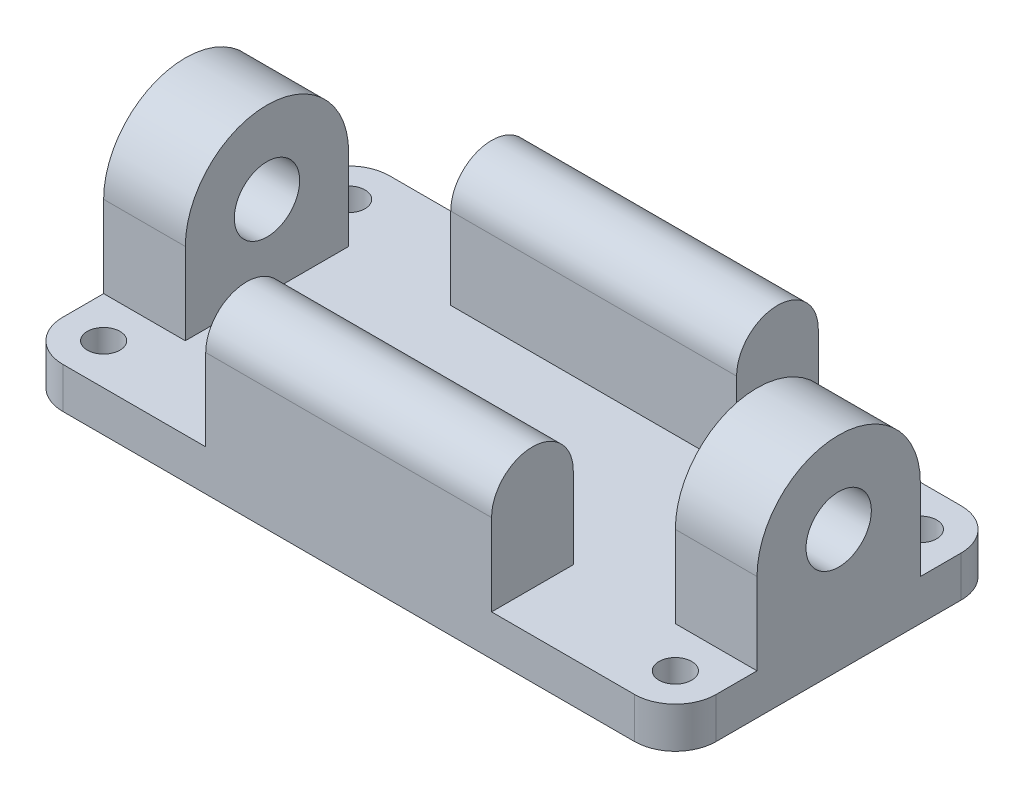
SolidWorks part; units mm, degrees
material "Plain Carbon Steel"
ref_plane "Front Plane" through (0, 0, 0) normal (0, 0, 1) x (1, 0, 0)
ref_plane "Top Plane" through (0, 0, 0) normal (0, 1, 0) x (1, 0, 0)
ref_plane "Right Plane" through (0, 0, 0) normal (1, 0, 0) x (0, 0, -1)
sketch "Base Plate Sketch" plane through (0, 0, 0) normal (0, 1, 0) x (1, 0, 0)
  line L1 (-35, -20) -> (35, -20)
  line L2 (-40, -15) -> (-40, 15)
  line L3 (-35, 20) -> (35, 20)
  line L4 (40, -15) -> (40, 15)
  line L5 (-40, -20) -> (40, 20) construction
  line L6 (-40, 20) -> (40, -20) construction
  arc A0 (35, 20) -> (40, 15) centre (35, 15) cw
  arc A1 (35, -20) -> (40, -15) centre (35, -15) ccw
  arc A2 (-35, -20) -> (-40, -15) centre (-35, -15) cw
  arc A3 (-40, 15) -> (-35, 20) centre (-35, 15) cw
  point P0 (0, 0)
  dimension "D3" = 5
  dimension "D1" = 80
  dimension "D2" = 40
extrude "Base Plate" add sketch "Base Plate Sketch" along normal blind 5
hole_wizard "Mounting Holes Ø4 Thru" positions "3DSketch1" profile "Sketch2" hole size "Ø4.0" standard "ANSI Metric" end condition through all
sketch3d "3DSketch1"
  arc A0 (-35, 5, -20) -> (-40, 5, -15) centre (-35, 5, -15) ccw construction
  arc A1 (40, 5, -15) -> (35, 5, -20) centre (35, 5, -15) ccw construction
  arc A2 (-40, 5, 15) -> (-35, 5, 20) centre (-35, 5, 15) ccw construction
  arc A3 (35, 5, 20) -> (40, 5, 15) centre (35, 5, 15) ccw construction
  point P0 (-35, 5, -15)
  point P6 (-35, 10, -15)
  point P8 (35, 5, -15)
  point P10 (35, 5, 15)
  point P12 (-35, 5, 15)
  point P19 (35, 10, -15)
  point P26 (-35, 10, 15)
  point P31 (35, 10, 15)
sketch "Sketch2" plane through (-35, 5, -15) normal (1, 0, 0) x (0, 0, 1)
  line L0 (0, 0) -> (0, 5)
  line L1 (0, 5) -> (2, 5)
  line L2 (2, 5) -> (2, 0)
  line L5 (2, 0) -> (0, 0)
  line L11 (0, -6.35) -> (0, 107.95) construction
  dimension "Thru Hole Dia." = 4
  dimension "Thru Hole Depth" = 5
sketch "End Lug Sketch" plane through (40, 0, 0) normal (1, 0, 0) x (0, 0, -1)
  line L0 (-10, 15) -> (-10, 5)
  line L1 (-15, 5) -> (15, 5) construction
  line L2 (-10, 5) -> (10, 5)
  line L3 (10, 5) -> (10, 15)
  line L4 (-20, 5) -> (-20, 0) construction
  arc A0 (10, 15) -> (-10, 15) centre (0, 15) ccw
  circle A1 centre (0, 15) radius 4
  point P11 (0, 25)
  dimension "D4" = 8
  dimension "D1" = 20
  dimension "D2" = 10
  dimension "D3" = 25
extrude "End Lug" add sketch "End Lug Sketch" against normal blind 10
mirror "End Lug Mirror" about plane through (0, 0, 0) normal (1, 0, 0) of "End Lug"
sketch "Guide Rail Sketch" plane through (0, 0, 0) normal (1, 0, 0) x (0, 0, -1)
  line L0 (-20, 5) -> (-20, 15)
  line L1 (-10, 15) -> (-10, 5)
  line L2 (-10, 5) -> (-20, 5)
  line L3 (-15, 0) -> (15, 0) construction
  arc A0 (-10, 15) -> (-20, 15) centre (-15, 15) ccw
  dimension "D1" = 5
  dimension "D2" = 15
extrude "Guide Rail" add sketch "Guide Rail Sketch" along normal mid plane 35
mirror "Guide Rail Mirror" about plane through (0, 0, 0) normal (0, 0, 1) of "Guide Rail"
